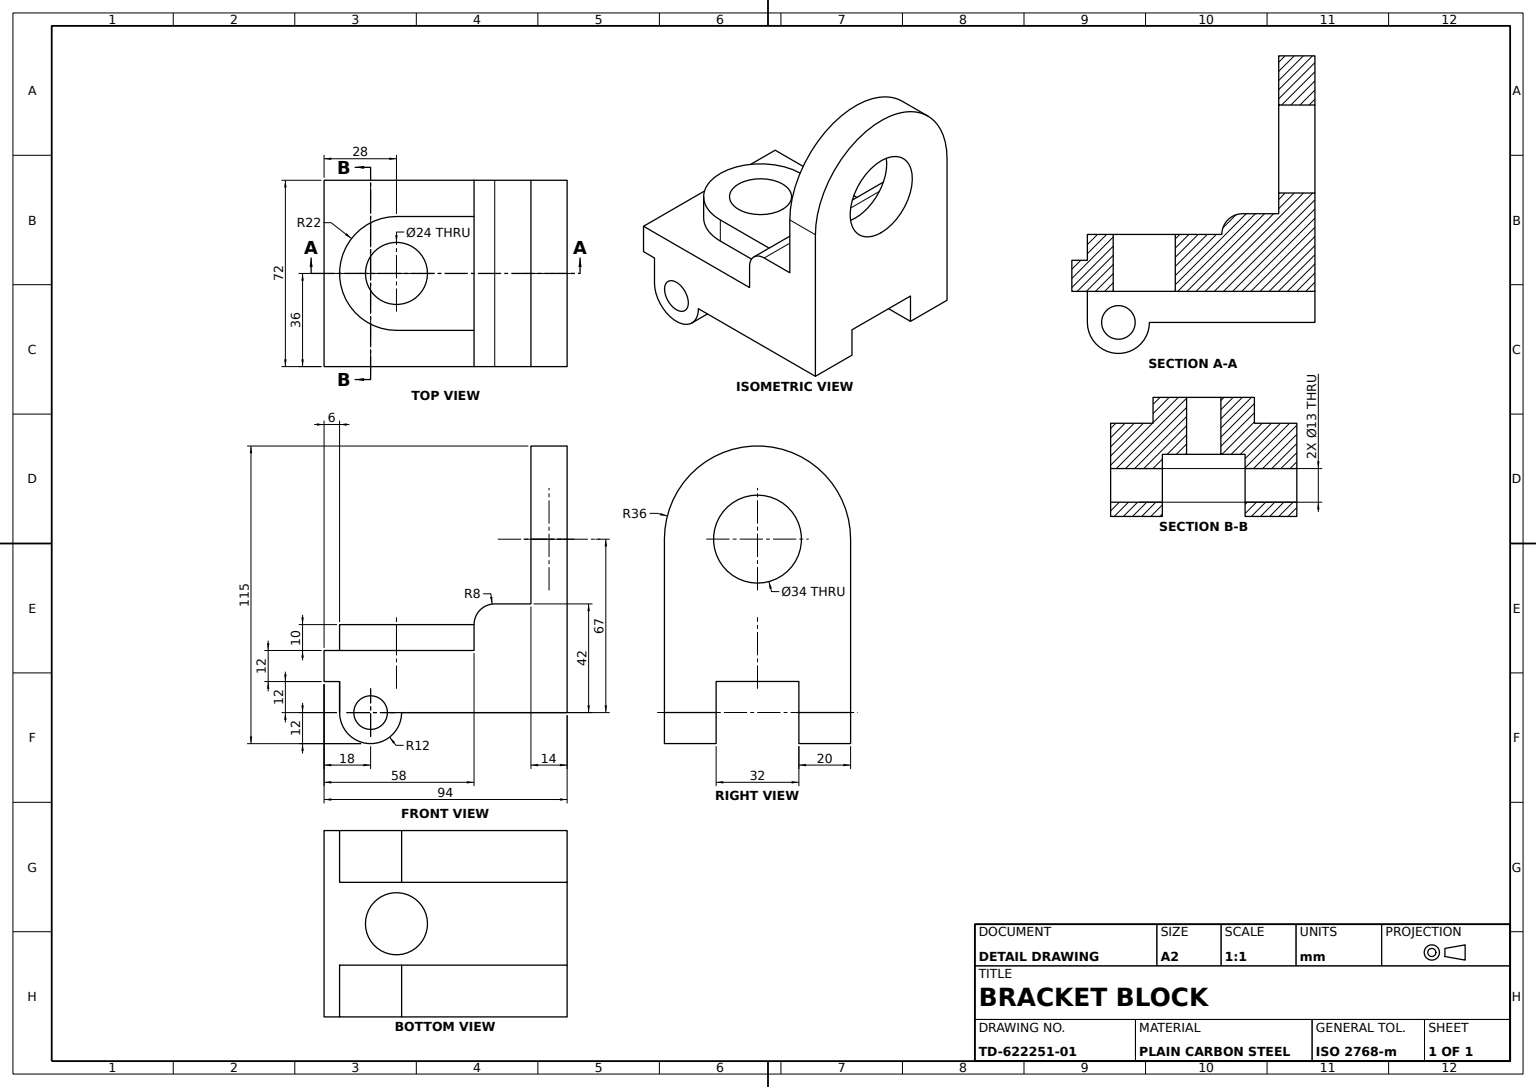
from build123d import *

# Parameters (mm, degrees)
BASE_BODY_PROFILE_R   = 6.5
BASE_BODY_DEPTH       = 36
POCKET_32X20_SKETCH_W = 32
POCKET_32X20_SKETCH_H = 24
POCKET_32X20_DEPTH    = 110.840793879
LUG_ROUNDED_TOP_DEPTH = 14
LUG_BORE_34_REACH     = 128.4
LUG_BORE_SKETCH_R     = 17
BOSS_10MM_DEPTH       = 10
BOSS_BORE_SKETCH_R    = 12
BOSS_BORE_24_DEPTH    = 123.036879672


with BuildPart() as part:
    # Base Body Profile → Base Body (new, symmetric)
    with BuildSketch(Plane.XY):
        with BuildLine():
            Line((0, -12), (0, 0))
            Line((0, 0), (0, 55))
            Line((0, 55), (-14, 55))
            Line((-14, 55), (-14, 30))
            Line((-14, 30), (-28, 30))
            ThreePointArc((-28, 30), (-33.656854249, 27.656854249), (-36, 22))
            Line((-36, 22), (-36, 12))
            Line((-36, 12), (-94, 12))
            Line((-94, 12), (-94, 0))
            Line((-94, 0), (-88, 0))
            Line((-88, 0), (-88, -12))
            ThreePointArc((-88, -12), (-76, -24), (-64, -12))
            Line((-64, -12), (0, -12))
        make_face()
        with Locations((-76, -12)):
            Circle(BASE_BODY_PROFILE_R, mode=Mode.SUBTRACT)
    extrude(amount=BASE_BODY_DEPTH, both=True)

    # Pocket 32x20 Sketch → Pocket 32x20 (cut, through all)
    with BuildSketch(Plane.ZY.offset(88)):
        with Locations((0, -12)):
            Rectangle(POCKET_32X20_SKETCH_W, POCKET_32X20_SKETCH_H)
    extrude(amount=-POCKET_32X20_DEPTH, mode=Mode.SUBTRACT)

    # Lug Rounded Top Sketch → Lug Rounded Top (add)
    with BuildSketch(Plane(origin=(0, 0, 0), x_dir=(0, 0, -1), z_dir=(1, 0, 0))):
        with BuildLine():
            Line((-36, 55), (36, 55))
            ThreePointArc((36, 55), (0, 91), (-36, 55))
        make_face()
    extrude(amount=-LUG_ROUNDED_TOP_DEPTH)

    # Lug Bore Sketch → Lug Bore Ø34 (cut, up to next)
    with BuildSketch(Plane.ZY.offset(14), mode=Mode.PRIVATE) as lug_bore_34_sk1:
        with Locations(Location((0, 55, 0), (0, 0, 270))):
            Circle(LUG_BORE_SKETCH_R)
    lug_bore_34_tool1 = extrude(lug_bore_34_sk1.sketch, amount=-LUG_BORE_34_REACH, mode=Mode.PRIVATE) & part.part
    add(lug_bore_34_tool1.solids().sort_by_distance((-14, 55, 0))[0], mode=Mode.SUBTRACT)

    # Boss Profile 44x30 → Boss 10mm (add)
    with BuildSketch(Plane(origin=(0, 12, 0), x_dir=(1, 0, 0), z_dir=(0, 1, 0))):
        with BuildLine():
            Line((-66, 22), (-36, 22))
            Line((-36, 22), (-36, -22))
            Line((-36, -22), (-66, -22))
            ThreePointArc((-66, -22), (-88, 0), (-66, 22))
        make_face()
    extrude(amount=BOSS_10MM_DEPTH)

    # Boss Bore Sketch → Boss Bore Ø24 (cut, through all)
    with BuildSketch(Plane(origin=(0, 22, 0), x_dir=(1, 0, 0), z_dir=(0, 1, 0))):
        with Locations(Location((-66, 0, 0), (0, 0, 180))):
            Circle(BOSS_BORE_SKETCH_R)
    extrude(amount=-BOSS_BORE_24_DEPTH, mode=Mode.SUBTRACT)


solid = part.part
